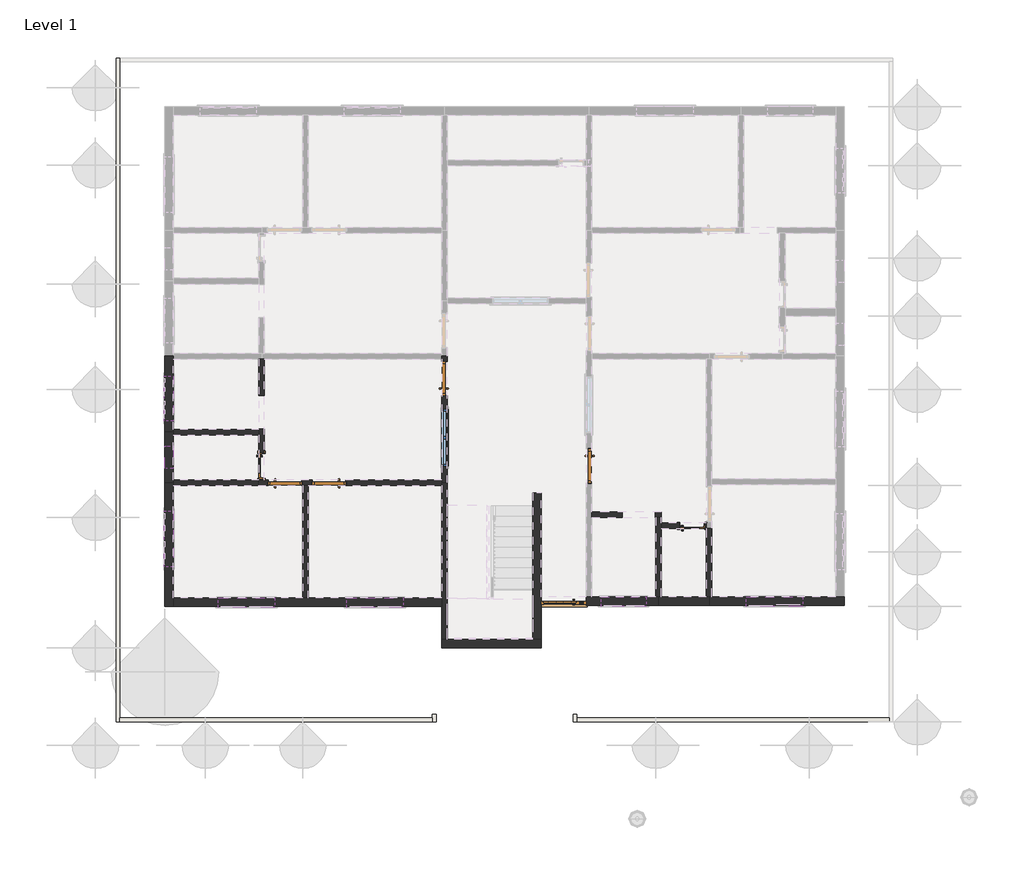
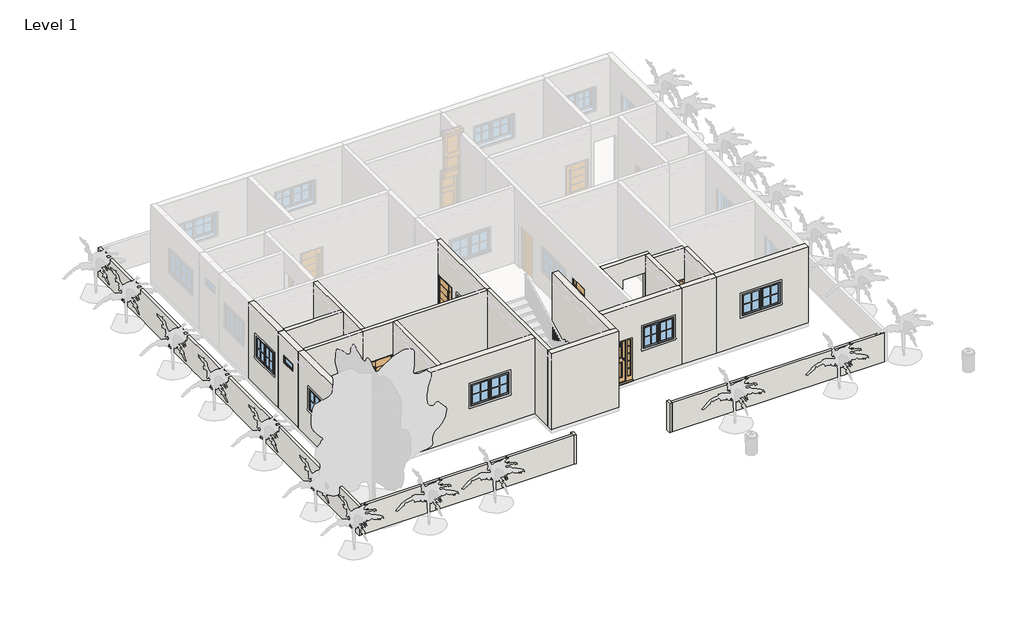
# One storey, part 1 of 5: 25 walls, 8 windows, 7 doors.
"""IFC4 building model written with IfcOpenShell, lengths in millimetres."""

from ifc_helpers import new_model, si_unit, frame, origin, origin_with_axes, place, context, project, spatial, polyline, outline, extrude, faceted_brep, transform, mapped, element, save
from components import door_3_ad1505b7, door_3_44036f4b, extsgl_w_side_panel_4_38b62cc9, door_c5a180fb, fixed_2_d9cafb20, m_window_awning_double_horizontal_4_0c6a2509, m_window_awning_double_horizontal_5_7c720334, m_window_awning_double_horizontal_5_337400f2

model = new_model("IFC4")

# Units and contexts
model_context = context("Model", 3, world=origin())
ifc_project = project(units=[si_unit("LENGTHUNIT", "METRE", prefix="MILLI")], contexts=[model_context])

# Site, building, storey
site = spatial("IfcSite", under=ifc_project)
building = spatial("IfcBuilding", under=site)
storey = spatial("IfcBuildingStorey", under=building, Name="Level 1", Elevation=0.0)

# Doors
placement = place(None, origin())
door_3_shape = door_3_ad1505b7(model_context)
element("IfcDoor", 1, ObjectType="3'", at=placement, inside=storey, context=model_context, shape_type="MappedRepresentation", body=[
    mapped(door_3_shape, transform((-17435.4847893, 15964.9922903, 0.0), x_axis=(0.0, 1.0, 0.0), y_axis=(-1.0, 0.0, 0.0), z_axis=(0.0, 0.0, 1.0))),
])
element("IfcDoor", 2, ObjectType="3'", at=placement, inside=storey, context=model_context, shape_type="MappedRepresentation", body=[
    mapped(door_3_shape, transform((-20559.6847893, 13145.5922903, 0.0), x_axis=(-1.0, 0.0, 0.0), y_axis=(0.0, -1.0, 0.0), z_axis=(0.0, 0.0, 1.0))),
])
element("IfcDoor", 3, ObjectType="3'", at=placement, inside=storey, context=model_context, shape_type="MappedRepresentation", body=[
    mapped(door_3_shape, transform((-13523.8847893, 13602.7922903, 0.0), x_axis=(0.0, -1.0, 0.0), y_axis=(1.0, 0.0, 0.0), z_axis=(0.0, 0.0, 1.0))),
])
door_3_2_shape = door_3_44036f4b(model_context)
element("IfcDoor", 4, ObjectType="3'", at=placement, inside=storey, context=model_context, shape_type="MappedRepresentation", body=[
    mapped(door_3_2_shape, transform((-21753.4847893, 13145.5922903, 0.0), x_axis=(1.0, 0.0, 0.0), y_axis=(0.0, 1.0, 0.0), z_axis=(0.0, 0.0, 1.0))),
])
extsgl_w_side_panel_4_shape = extsgl_w_side_panel_4_38b62cc9(model_context)
element("IfcDoor", 5, ObjectType="ExtSgl w Side Panel : 4'", at=placement, inside=storey, context=model_context, shape_type="MappedRepresentation", body=[
    mapped(extsgl_w_side_panel_4_shape, transform((-14429.0847893, 9932.4922903, 0.0), x_axis=(-1.0, 0.0, 0.0), y_axis=(0.0, -1.0, 0.0), z_axis=(0.0, 0.0, 1.0))),
])
door_shape = door_c5a180fb(model_context)
element("IfcDoor", 6, ObjectType="M_Door-Interior-Single-2_Panel-Wood : 2'2\"", at=placement, inside=storey, context=model_context, shape_type="MappedRepresentation", body=[
    mapped(door_shape, transform((-22391.6597893, 13602.7922903, 0.0), x_axis=(0.0, -1.0, 0.0), y_axis=(1.0, 0.0, 0.0), z_axis=(0.0, 0.0, 1.0))),
])
element("IfcDoor", 7, ObjectType="M_Door-Interior-Single-2_Panel-Wood : 2'2\"", at=placement, inside=storey, context=model_context, shape_type="MappedRepresentation", body=[
    mapped(door_shape, transform((-10729.8847893, 11974.0172903, 0.0), x_axis=(1.0, 0.0, 0.0), y_axis=(0.0, 1.0, 0.0), z_axis=(0.0, 0.0, 1.0))),
])

# Walls
element("IfcWall", 8, ObjectType="Generic - 4\"", at=placement, inside=storey, context=model_context, shape_type="Brep", body=[
    faceted_brep([(-26325.4847893, 24651.7922903, -152.4), (-26325.4847893, 6668.5922903, -152.4), (-26325.4847893, 6668.5922903, 1066.8), (-26325.4847893, 24651.7922903, 1066.8), (-26223.8847893, 24651.7922903, -152.4), (-26223.8847893, 24651.7922903, 1066.8), (-26223.8847893, 24550.1922903, 1066.8), (-26223.8847893, 6770.1922903, 1066.8), (-26223.8847893, 6668.5922903, 1066.8), (-26223.8847893, 6668.5922903, -152.4), (-26223.8847893, 6770.1922903, -152.4), (-26223.8847893, 24550.1922903, -152.4)], [[[0, 1, 2, 3]], [[4, 5, 6, 7, 8, 9, 10, 11]], [[1, 0, 4, 11, 10, 9]], [[3, 2, 8, 7, 6, 5]], [[2, 1, 9, 8]], [[0, 3, 5, 4]]]),
])
element("IfcWall", 9, ObjectType="Generic - 4\"", at=placement, inside=storey, context=model_context, shape_type="SweptSolid", body=[
    extrude(outline(polyline([(-17765.6847893, 6668.5922903), (-26223.8847893, 6668.5922903), (-26223.8847893, 6770.1922903), (-17765.6847893, 6770.1922903), (-17765.6847893, 6668.5922903)])), frame((0.0, 0.0, -152.4), z_axis=(0.0, 0.0, 1.0), x_axis=(1.0, 0.0, 0.0)), (0.0, 0.0, 1.0), 1219.2),
])
element("IfcWall", 10, ObjectType="Generic - 4\"", at=placement, inside=storey, context=model_context, shape_type="Brep", body=[
    faceted_brep([(-17664.0847893, 6668.5922903, -152.4), (-17664.0847893, 6871.7922903, -152.4), (-17664.0847893, 6871.7922903, 1066.8), (-17664.0847893, 6668.5922903, 1066.8), (-17765.6847893, 6668.5922903, -152.4), (-17765.6847893, 6668.5922903, 1066.8), (-17765.6847893, 6770.1922903, 1066.8), (-17765.6847893, 6871.7922903, 1066.8), (-17765.6847893, 6871.7922903, -152.4), (-17765.6847893, 6770.1922903, -152.4)], [[[0, 1, 2, 3]], [[4, 5, 6, 7, 8, 9]], [[1, 0, 4, 9, 8]], [[2, 1, 8, 7]], [[3, 2, 7, 6, 5]], [[0, 3, 5, 4]]]),
])
element("IfcWall", 11, ObjectType="Generic - 4\"", at=placement, inside=storey, context=model_context, shape_type="SweptSolid", body=[
    extrude(outline(polyline([(-13854.0847893, 6770.1922903), (-5395.8847893, 6770.1922903), (-5395.8847893, 6668.5922903), (-13854.0847893, 6668.5922903), (-13854.0847893, 6770.1922903)])), frame((0.0, 0.0, -152.4), z_axis=(0.0, 0.0, 1.0), x_axis=(1.0, 0.0, 0.0)), (0.0, 0.0, 1.0), 1219.2),
])
element("IfcWall", 12, ObjectType="Generic - 4\"", at=placement, inside=storey, context=model_context, shape_type="Brep", body=[
    faceted_brep([(-13955.6847893, 6871.7922903, -152.4), (-13955.6847893, 6668.5922903, -152.4), (-13955.6847893, 6668.5922903, 1066.8), (-13955.6847893, 6871.7922903, 1066.8), (-13854.0847893, 6871.7922903, -152.4), (-13854.0847893, 6871.7922903, 1066.8), (-13854.0847893, 6770.1922903, 1066.8), (-13854.0847893, 6668.5922903, 1066.8), (-13854.0847893, 6668.5922903, -152.4), (-13854.0847893, 6770.1922903, -152.4)], [[[0, 1, 2, 3]], [[4, 5, 6, 7, 8, 9]], [[1, 0, 4, 9, 8]], [[3, 2, 7, 6, 5]], [[0, 3, 5, 4]], [[2, 1, 8, 7]]]),
])
element("IfcWall", 13, ObjectType="Generic - 6\"", at=placement, inside=storey, context=model_context, shape_type="Brep", body=[
    faceted_brep([(-24776.0847893, 13069.3922903, 0.0), (-22477.3847893, 13069.3922903, 0.0), (-22477.3847893, 13069.3922903, 3200.4), (-24776.0847893, 13069.3922903, 3200.4), (-24776.0847893, 13221.7922903, 0.0), (-24776.0847893, 13221.7922903, 3200.4), (-22477.3847893, 13221.7922903, 3200.4), (-22477.3847893, 13221.7922903, 0.0), (-24776.0847893, 13145.5922903, 0.0), (-24776.0847893, 13145.5922903, 3200.4)], [[[0, 1, 2, 3]], [[4, 5, 6, 7]], [[1, 0, 8, 4, 7]], [[2, 1, 7, 6]], [[3, 2, 6, 5, 9]], [[0, 3, 9, 5, 4, 8]]]),
])
element("IfcWall", 14, ObjectType="Generic - 6\"", at=placement, inside=storey, context=model_context, shape_type="Brep", body=[
    faceted_brep([(-22464.6847893, 13221.7922903, 3200.4), (-22464.6847893, 14440.9922903, 3200.4), (-22464.6847893, 14593.3922903, 3200.4), (-22464.6847893, 16498.3922903, 3200.4), (-22464.6847893, 16498.3922903, 0.0), (-22464.6847893, 15507.100075, 0.0), (-22464.6847893, 15507.100075, 2438.4), (-22464.6847893, 14599.1617976, 2438.4), (-22464.6847893, 14599.1617976, 0.0), (-22464.6847893, 14593.3922903, 0.0), (-22464.6847893, 14440.9922903, 0.0), (-22464.6847893, 13957.9922903, 0.0), (-22464.6847893, 13957.9922903, 1853.8), (-22464.6847893, 13247.5922903, 1853.8), (-22464.6847893, 13247.5922903, 0.0), (-22464.6847893, 13221.7922903, 0.0), (-22312.2847893, 16498.3922903, 3200.4), (-22312.2847893, 13221.7922903, 3200.4), (-22312.2847893, 13221.7922903, 0.0), (-22312.2847893, 13247.5922903, 0.0), (-22312.2847893, 13247.5922903, 1853.8), (-22312.2847893, 13957.9922903, 1853.8), (-22312.2847893, 13957.9922903, 0.0), (-22312.2847893, 14599.1617976, 0.0), (-22312.2847893, 14599.1617976, 2438.4), (-22312.2847893, 15507.100075, 2438.4), (-22312.2847893, 15507.100075, 0.0), (-22312.2847893, 16498.3922903, 0.0), (-22388.4847893, 16498.3922903, 0.0), (-22388.4847893, 16498.3922903, 3200.4)], [[[0, 1, 2, 3, 4, 5, 6, 7, 8, 9, 10, 11, 12, 13, 14, 15]], [[16, 17, 18, 19, 20, 21, 22, 23, 24, 25, 26, 27]], [[18, 15, 14, 19]], [[8, 23, 22, 11, 10, 9]], [[4, 28, 27, 26, 5]], [[3, 2, 1, 0, 17, 16, 29]], [[4, 3, 29, 16, 27, 28]], [[0, 15, 18, 17]], [[13, 20, 19, 14]], [[20, 13, 12, 21]], [[21, 12, 11, 22]], [[6, 25, 24, 7]], [[25, 6, 5, 26]], [[7, 24, 23, 8]]]),
])
element("IfcWall", 15, ObjectType="Generic - 6\"", at=placement, inside=storey, context=model_context, shape_type="Brep", body=[
    faceted_brep([(-24776.0847893, 14440.9922903, 0.0), (-22464.6847893, 14440.9922903, 0.0), (-22464.6847893, 14440.9922903, 3200.4), (-24776.0847893, 14440.9922903, 3200.4), (-24776.0847893, 14593.3922903, 0.0), (-24776.0847893, 14593.3922903, 3200.4), (-22464.6847893, 14593.3922903, 3200.4), (-22464.6847893, 14593.3922903, 0.0), (-24776.0847893, 14517.1922903, 0.0), (-24776.0847893, 14517.1922903, 3200.4)], [[[0, 1, 2, 3]], [[4, 5, 6, 7]], [[1, 0, 8, 4, 7]], [[3, 2, 6, 5, 9]], [[0, 3, 9, 5, 4, 8]], [[2, 1, 7, 6]]]),
])
element("IfcWall", 16, ObjectType="Generic - 6\"", at=placement, inside=storey, context=model_context, shape_type="SweptSolid", body=[
    extrude(outline(polyline([(-21118.4847893, 13069.3922903), (-21118.4847893, 10021.3922903), (-21270.8847893, 10021.3922903), (-21270.8847893, 13069.3922903), (-21118.4847893, 13069.3922903)])), origin_with_axes(), (0.0, 0.0, 1.0), 3200.4),
])
element("IfcWall", 17, ObjectType="Generic - 6\"", at=placement, inside=storey, context=model_context, shape_type="Brep", body=[
    faceted_brep([(-11568.0847893, 12205.7922903, 0.0), (-11568.0847893, 12205.7922903, 3200.4), (-11720.4847893, 12205.7922903, 3200.4), (-13447.6847893, 12205.7922903, 3200.4), (-13447.6847893, 12205.7922903, 0.0), (-12628.6631671, 12205.7922903, 0.0), (-12628.6631671, 12205.7922903, 2438.4), (-11726.8987952, 12205.7922903, 2438.4), (-11726.8987952, 12205.7922903, 0.0), (-11720.4847893, 12205.7922903, 0.0), (-11568.0847893, 12358.1922903, 3200.4), (-11568.0847893, 12358.1922903, 0.0), (-11726.8987952, 12358.1922903, 0.0), (-11726.8987952, 12358.1922903, 2438.4), (-12628.6631671, 12358.1922903, 2438.4), (-12628.6631671, 12358.1922903, 0.0), (-13447.6847893, 12358.1922903, 0.0), (-13447.6847893, 12358.1922903, 3200.4)], [[[0, 1, 2, 3, 4, 5, 6, 7, 8, 9]], [[10, 11, 12, 13, 14, 15, 16, 17]], [[4, 16, 15, 5]], [[11, 0, 9, 8, 12]], [[3, 2, 1, 10, 17]], [[4, 3, 17, 16]], [[1, 0, 11, 10]], [[6, 14, 13, 7]], [[14, 6, 5, 15]], [[7, 13, 12, 8]]]),
])
element("IfcWall", 18, ObjectType="Generic - 6\"", at=placement, inside=storey, context=model_context, shape_type="Brep", body=[
    faceted_brep([(-11720.4847893, 12205.7922903, 0.0), (-11720.4847893, 10046.7922903, 0.0), (-11720.4847893, 10046.7922903, 3200.4), (-11720.4847893, 12205.7922903, 3200.4), (-11568.0847893, 12205.7922903, 0.0), (-11568.0847893, 12205.7922903, 3200.4), (-11568.0847893, 12053.3922903, 3200.4), (-11568.0847893, 11900.9922903, 3200.4), (-11568.0847893, 10046.7922903, 3200.4), (-11568.0847893, 10046.7922903, 0.0), (-11568.0847893, 11900.9922903, 0.0), (-11568.0847893, 12053.3922903, 0.0), (-11644.2847893, 10046.7922903, 0.0), (-11644.2847893, 10046.7922903, 3200.4)], [[[0, 1, 2, 3]], [[4, 5, 6, 7, 8, 9, 10, 11]], [[1, 0, 4, 11, 10, 9, 12]], [[3, 2, 13, 8, 7, 6, 5]], [[0, 3, 5, 4]], [[2, 1, 12, 9, 8, 13]]]),
])
element("IfcWall", 19, ObjectType="Generic - 6\"", at=placement, inside=storey, context=model_context, shape_type="Brep", body=[
    faceted_brep([(-10348.8847893, 11900.9922903, 3200.4), (-11568.0847893, 11900.9922903, 3200.4), (-11568.0847893, 11900.9922903, 0.0), (-11085.0847893, 11900.9922903, 0.0), (-11085.0847893, 11900.9922903, 1853.8), (-10374.6847893, 11900.9922903, 1853.8), (-10374.6847893, 11900.9922903, 0.0), (-10348.8847893, 11900.9922903, 0.0), (-11568.0847893, 12053.3922903, 3200.4), (-10348.8847893, 12053.3922903, 3200.4), (-10348.8847893, 12053.3922903, 0.0), (-10374.6847893, 12053.3922903, 0.0), (-10374.6847893, 12053.3922903, 1853.8), (-11085.0847893, 12053.3922903, 1853.8), (-11085.0847893, 12053.3922903, 0.0), (-11568.0847893, 12053.3922903, 0.0), (-10348.8847893, 11913.6922903, 0.0), (-10348.8847893, 11913.6922903, 3200.4)], [[[0, 1, 2, 3, 4, 5, 6, 7]], [[8, 9, 10, 11, 12, 13, 14, 15]], [[2, 15, 14, 3]], [[10, 16, 7, 6, 11]], [[1, 0, 17, 9, 8]], [[0, 7, 16, 10, 9, 17]], [[2, 1, 8, 15]], [[5, 12, 11, 6]], [[12, 5, 4, 13]], [[13, 4, 3, 14]]]),
])
element("IfcWall", 20, ObjectType="Generic - 6\"", at=placement, inside=storey, context=model_context, shape_type="Brep", body=[
    faceted_brep([(-17511.6847893, 13145.5922903, 0.0), (-17511.6847893, 13145.5922903, 3200.4), (-17511.6847893, 13221.7922903, 3200.4), (-17511.6847893, 16498.3922903, 3200.4), (-17511.6847893, 16574.5922903, 3200.4), (-17511.6847893, 16574.5922903, 0.0), (-17511.6847893, 16498.3922903, 0.0), (-17511.6847893, 16422.1922903, 0.0), (-17511.6847893, 16422.1922903, 1828.8), (-17511.6847893, 15507.7922903, 1828.8), (-17511.6847893, 15507.7922903, 0.0), (-17511.6847893, 13221.7922903, 0.0), (-17511.6847893, 13602.7922903, 1814.4), (-17511.6847893, 13602.7922903, 900.0), (-17511.6847893, 15126.7922903, 900.0), (-17511.6847893, 15126.7922903, 1814.4), (-17359.2847893, 13145.5922903, 3200.4), (-17359.2847893, 13145.5922903, 0.0), (-17359.2847893, 15507.7922903, 0.0), (-17359.2847893, 15507.7922903, 1828.8), (-17359.2847893, 16422.1922903, 1828.8), (-17359.2847893, 16422.1922903, 0.0), (-17359.2847893, 16574.5922903, 0.0), (-17359.2847893, 16574.5922903, 3200.4), (-17359.2847893, 13602.7922903, 1814.4), (-17359.2847893, 15126.7922903, 1814.4), (-17359.2847893, 15126.7922903, 900.0), (-17359.2847893, 13602.7922903, 900.0), (-17414.6847893, 16422.1922903, 0.0), (-17414.6847893, 16437.1922903, 0.0), (-17491.6847893, 16437.1922903, 0.0), (-17491.6847893, 16422.1922903, 0.0), (-17491.6847893, 15507.7922903, 0.0), (-17491.6847893, 15492.7922903, 0.0), (-17414.6847893, 15492.7922903, 0.0), (-17414.6847893, 15507.7922903, 0.0), (-17414.6847893, 15507.7922903, 1828.8), (-17414.6847893, 16422.1922903, 1828.8), (-17491.6847893, 16422.1922903, 1828.8), (-17491.6847893, 15507.7922903, 1828.8), (-17491.6847893, 15492.7922903, 1843.8), (-17491.6847893, 16437.1922903, 1843.8), (-17414.6847893, 16437.1922903, 1843.8), (-17414.6847893, 15492.7922903, 1843.8)], [[[0, 1, 2, 3, 4, 5, 6, 7, 8, 9, 10, 11], [12, 13, 14, 15]], [[16, 17, 18, 19, 20, 21, 22, 23], [24, 25, 26, 27]], [[5, 22, 21, 28, 29, 30, 31, 7, 6]], [[17, 0, 11, 10, 32, 33, 34, 35, 18]], [[1, 0, 17, 16]], [[4, 3, 2, 1, 16, 23]], [[5, 4, 23, 22]], [[19, 36, 37, 20]], [[8, 38, 39, 9]], [[20, 37, 28, 21]], [[38, 8, 7, 31]], [[36, 19, 18, 35]], [[9, 39, 32, 10]], [[40, 41, 42, 43]], [[42, 41, 30, 29]], [[37, 36, 35, 34, 43, 42, 29, 28]], [[40, 43, 34, 33]], [[39, 38, 31, 30, 41, 40, 33, 32]], [[12, 15, 25, 24]], [[15, 14, 26, 25]], [[14, 13, 27, 26]], [[13, 12, 24, 27]]]),
])
element("IfcWall", 21, ObjectType="Generic - 6\"", at=placement, inside=storey, context=model_context, shape_type="Brep", body=[
    faceted_brep([(-17511.6847893, 13145.5922903, 0.0), (-17511.6847893, 13069.3922903, 0.0), (-17511.6847893, 10021.3922903, 0.0), (-17511.6847893, 9792.7922903, 0.0), (-17511.6847893, 8903.7922903, 0.0), (-17511.6847893, 8903.7922903, 3200.4), (-17511.6847893, 9792.7922903, 3200.4), (-17511.6847893, 10021.3922903, 3200.4), (-17511.6847893, 13069.3922903, 3200.4), (-17511.6847893, 13145.5922903, 3200.4), (-17359.2847893, 13145.5922903, 0.0), (-17359.2847893, 13145.5922903, 3200.4), (-17359.2847893, 8903.7922903, 3200.4), (-17359.2847893, 8903.7922903, 0.0)], [[[0, 1, 2, 3, 4, 5, 6, 7, 8, 9]], [[10, 11, 12, 13]], [[4, 3, 2, 1, 0, 10, 13]], [[9, 8, 7, 6, 5, 12, 11]], [[0, 9, 11, 10]], [[5, 4, 13, 12]]]),
])
element("IfcWall", 22, ObjectType="Generic - 6\"", at=placement, inside=storey, context=model_context, shape_type="Brep", body=[
    faceted_brep([(-17511.6847893, 13069.3922903, 3200.4), (-21118.4847893, 13069.3922903, 3200.4), (-21270.8847893, 13069.3922903, 3200.4), (-22477.3847893, 13069.3922903, 3200.4), (-22477.3847893, 13069.3922903, 0.0), (-22210.6847893, 13069.3922903, 0.0), (-22210.6847893, 13069.3922903, 1828.8), (-21296.2847893, 13069.3922903, 1828.8), (-21296.2847893, 13069.3922903, 0.0), (-21270.8847893, 13069.3922903, 0.0), (-21118.4847893, 13069.3922903, 0.0), (-21016.8847893, 13069.3922903, 0.0), (-21016.8847893, 13069.3922903, 1828.8), (-20102.4847893, 13069.3922903, 1828.8), (-20102.4847893, 13069.3922903, 0.0), (-17511.6847893, 13069.3922903, 0.0), (-22477.3847893, 13221.7922903, 3200.4), (-22464.6847893, 13221.7922903, 3200.4), (-22312.2847893, 13221.7922903, 3200.4), (-17511.6847893, 13221.7922903, 3200.4), (-17511.6847893, 13221.7922903, 0.0), (-20102.4847893, 13221.7922903, 0.0), (-20102.4847893, 13221.7922903, 1828.8), (-21016.8847893, 13221.7922903, 1828.8), (-21016.8847893, 13221.7922903, 0.0), (-21296.2847893, 13221.7922903, 0.0), (-21296.2847893, 13221.7922903, 1828.8), (-22210.6847893, 13221.7922903, 1828.8), (-22210.6847893, 13221.7922903, 0.0), (-22312.2847893, 13221.7922903, 0.0), (-22464.6847893, 13221.7922903, 0.0), (-22477.3847893, 13221.7922903, 0.0), (-17511.6847893, 13145.5922903, 0.0), (-20102.4847893, 13089.3922903, 0.0), (-20087.4847893, 13089.3922903, 0.0), (-20087.4847893, 13166.3922903, 0.0), (-20102.4847893, 13166.3922903, 0.0), (-21296.2847893, 13089.3922903, 0.0), (-21281.2847893, 13089.3922903, 0.0), (-21281.2847893, 13166.3922903, 0.0), (-21296.2847893, 13166.3922903, 0.0), (-21016.8847893, 13166.3922903, 0.0), (-21031.8847893, 13166.3922903, 0.0), (-21031.8847893, 13089.3922903, 0.0), (-21016.8847893, 13089.3922903, 0.0), (-22210.6847893, 13166.3922903, 0.0), (-22225.6847893, 13166.3922903, 0.0), (-22225.6847893, 13089.3922903, 0.0), (-22210.6847893, 13089.3922903, 0.0), (-17511.6847893, 13145.5922903, 3200.4), (-22210.6847893, 13166.3922903, 1828.8), (-21296.2847893, 13166.3922903, 1828.8), (-22210.6847893, 13089.3922903, 1828.8), (-21296.2847893, 13089.3922903, 1828.8), (-21281.2847893, 13089.3922903, 1843.8), (-22225.6847893, 13089.3922903, 1843.8), (-22225.6847893, 13166.3922903, 1843.8), (-21281.2847893, 13166.3922903, 1843.8), (-20102.4847893, 13166.3922903, 1828.8), (-21016.8847893, 13166.3922903, 1828.8), (-21016.8847893, 13089.3922903, 1828.8), (-20102.4847893, 13089.3922903, 1828.8), (-20087.4847893, 13089.3922903, 1843.8), (-21031.8847893, 13089.3922903, 1843.8), (-21031.8847893, 13166.3922903, 1843.8), (-20087.4847893, 13166.3922903, 1843.8)], [[[0, 1, 2, 3, 4, 5, 6, 7, 8, 9, 10, 11, 12, 13, 14, 15]], [[16, 17, 18, 19, 20, 21, 22, 23, 24, 25, 26, 27, 28, 29, 30, 31]], [[20, 32, 15, 14, 33, 34, 35, 36, 21]], [[8, 37, 38, 39, 40, 25, 24, 41, 42, 43, 44, 11, 10, 9]], [[4, 31, 30, 29, 28, 45, 46, 47, 48, 5]], [[3, 2, 1, 0, 49, 19, 18, 17, 16]], [[4, 3, 16, 31]], [[0, 15, 32, 20, 19, 49]], [[50, 27, 26, 51]], [[6, 52, 53, 7]], [[51, 26, 25, 40]], [[7, 53, 37, 8]], [[27, 50, 45, 28]], [[52, 6, 5, 48]], [[54, 55, 56, 57]], [[54, 57, 39, 38]], [[57, 56, 46, 45, 50, 51, 40, 39]], [[56, 55, 47, 46]], [[55, 54, 38, 37, 53, 52, 48, 47]], [[22, 58, 59, 23]], [[12, 60, 61, 13]], [[23, 59, 41, 24]], [[60, 12, 11, 44]], [[58, 22, 21, 36]], [[13, 61, 33, 14]], [[62, 63, 64, 65]], [[64, 63, 43, 42]], [[59, 58, 36, 35, 65, 64, 42, 41]], [[62, 65, 35, 34]], [[61, 60, 44, 43, 63, 62, 34, 33]]]),
])
element("IfcWall", 23, ObjectType="Generic - 6\"", at=placement, inside=storey, context=model_context, shape_type="Brep", body=[
    faceted_brep([(-10348.8847893, 11913.6922903, 0.0), (-10348.8847893, 10046.7922903, 0.0), (-10348.8847893, 10046.7922903, 3200.4), (-10348.8847893, 11913.6922903, 3200.4), (-10196.4847893, 11913.6922903, 0.0), (-10196.4847893, 11913.6922903, 3200.4), (-10196.4847893, 10046.7922903, 3200.4), (-10196.4847893, 10046.7922903, 0.0), (-10272.6847893, 10046.7922903, 0.0), (-10272.6847893, 10046.7922903, 3200.4)], [[[0, 1, 2, 3]], [[4, 5, 6, 7]], [[1, 0, 4, 7, 8]], [[3, 2, 9, 6, 5]], [[0, 3, 5, 4]], [[2, 1, 8, 7, 6, 9]]]),
])
element("IfcWall", 24, ObjectType="Generic - 9\"", at=placement, inside=storey, context=model_context, shape_type="Brep", body=[
    faceted_brep([(-24776.0847893, 9792.7922903, 0.0), (-17511.6847893, 9792.7922903, 0.0), (-17511.6847893, 9792.7922903, 3200.4), (-24776.0847893, 9792.7922903, 3200.4), (-23556.8847893, 9792.7922903, 2133.5570313), (-22032.8847893, 9792.7922903, 2133.5570313), (-22032.8847893, 9792.7922903, 1219.1570313), (-23556.8847893, 9792.7922903, 1219.1570313), (-20077.0847893, 9792.7922903, 2133.5570313), (-18553.0847893, 9792.7922903, 2133.5570313), (-18553.0847893, 9792.7922903, 1219.1570313), (-20077.0847893, 9792.7922903, 1219.1570313), (-24776.0847893, 10021.3922903, 0.0), (-24776.0847893, 10021.3922903, 3200.4), (-21270.8847893, 10021.3922903, 3200.4), (-21118.4847893, 10021.3922903, 3200.4), (-17511.6847893, 10021.3922903, 3200.4), (-17511.6847893, 10021.3922903, 0.0), (-21118.4847893, 10021.3922903, 0.0), (-21270.8847893, 10021.3922903, 0.0), (-23556.8847893, 10021.3922903, 2133.5570313), (-23556.8847893, 10021.3922903, 1219.1570313), (-22032.8847893, 10021.3922903, 1219.1570313), (-22032.8847893, 10021.3922903, 2133.5570313), (-20077.0847893, 10021.3922903, 2133.5570313), (-20077.0847893, 10021.3922903, 1219.1570313), (-18553.0847893, 10021.3922903, 1219.1570313), (-18553.0847893, 10021.3922903, 2133.5570313)], [[[0, 1, 2, 3], [4, 5, 6, 7], [8, 9, 10, 11]], [[12, 13, 14, 15, 16, 17, 18, 19], [20, 21, 22, 23], [24, 25, 26, 27]], [[1, 0, 12, 19, 18, 17]], [[3, 2, 16, 15, 14, 13]], [[0, 3, 13, 12]], [[2, 1, 17, 16]], [[21, 20, 4, 7]], [[22, 21, 7, 6]], [[23, 22, 6, 5]], [[20, 23, 5, 4]], [[25, 24, 8, 11]], [[26, 25, 11, 10]], [[27, 26, 10, 9]], [[24, 27, 9, 8]]]),
])
element("IfcWall", 25, ObjectType="Generic - 9\"", at=placement, inside=storey, context=model_context, shape_type="Brep", body=[
    faceted_brep([(-17511.6847893, 8675.1922903, 0.0), (-14819.2847893, 8675.1922903, 0.0), (-14819.2847893, 8675.1922903, 3200.4), (-17511.6847893, 8675.1922903, 3200.4), (-17511.6847893, 8903.7922903, 0.0), (-17511.6847893, 8903.7922903, 3200.4), (-17359.2847893, 8903.7922903, 3200.4), (-15047.8847893, 8903.7922903, 3200.4), (-14819.2847893, 8903.7922903, 3200.4), (-14819.2847893, 8903.7922903, 0.0), (-15047.8847893, 8903.7922903, 0.0), (-17359.2847893, 8903.7922903, 0.0)], [[[0, 1, 2, 3]], [[4, 5, 6, 7, 8, 9, 10, 11]], [[1, 0, 4, 11, 10, 9]], [[3, 2, 8, 7, 6, 5]], [[2, 1, 9, 8]], [[0, 3, 5, 4]]]),
])
element("IfcWall", 26, ObjectType="Generic - 9\"", at=placement, inside=storey, context=model_context, shape_type="Brep", body=[
    faceted_brep([(-14819.2847893, 8903.7922903, 0.0), (-14819.2847893, 9818.1922903, 0.0), (-14819.2847893, 10046.7922903, 0.0), (-14819.2847893, 12866.1922903, 0.0), (-14819.2847893, 12866.1922903, 3200.4), (-14819.2847893, 10046.7922903, 3200.4), (-14819.2847893, 9818.1922903, 3200.4), (-14819.2847893, 8903.7922903, 3200.4), (-15047.8847893, 8903.7922903, 0.0), (-15047.8847893, 8903.7922903, 3200.4), (-15047.8847893, 12866.1922903, 3200.4), (-15047.8847893, 12866.1922903, 0.0)], [[[0, 1, 2, 3, 4, 5, 6, 7]], [[8, 9, 10, 11]], [[3, 2, 1, 0, 8, 11]], [[4, 3, 11, 10]], [[7, 6, 5, 4, 10, 9]], [[0, 7, 9, 8]]]),
])
element("IfcWall", 27, ObjectType="Generic - 9\"", at=placement, inside=storey, context=model_context, shape_type="Brep", body=[
    faceted_brep([(-6615.0847893, 10046.7922903, 0.0), (-6843.6847893, 10046.7922903, 0.0), (-10196.4847893, 10046.7922903, 0.0), (-10272.6847893, 10046.7922903, 0.0), (-10272.6847893, 10046.7922903, 3200.4), (-10196.4847893, 10046.7922903, 3200.4), (-6843.6847893, 10046.7922903, 3200.4), (-6615.0847893, 10046.7922903, 3200.4), (-9263.0347893, 10046.7922903, 2133.5570313), (-9263.0347893, 10046.7922903, 1219.1570313), (-7739.0347893, 10046.7922903, 1219.1570313), (-7739.0347893, 10046.7922903, 2133.5570313), (-6615.0847893, 9818.1922903, 0.0), (-6615.0847893, 9818.1922903, 3200.4), (-10272.6847893, 9818.1922903, 3200.4), (-10272.6847893, 9818.1922903, 0.0), (-9263.0347893, 9818.1922903, 2133.5570313), (-7739.0347893, 9818.1922903, 2133.5570313), (-7739.0347893, 9818.1922903, 1219.1570313), (-9263.0347893, 9818.1922903, 1219.1570313)], [[[0, 1, 2, 3, 4, 5, 6, 7], [8, 9, 10, 11]], [[12, 13, 14, 15], [16, 17, 18, 19]], [[3, 2, 1, 0, 12, 15]], [[4, 3, 15, 14]], [[7, 6, 5, 4, 14, 13]], [[0, 7, 13, 12]], [[9, 8, 16, 19]], [[10, 9, 19, 18]], [[11, 10, 18, 17]], [[8, 11, 17, 16]]]),
])
element("IfcWall", 28, ObjectType="Generic - 9\"", at=placement, inside=storey, context=model_context, shape_type="Brep", body=[
    faceted_brep([(-10272.6847893, 10046.7922903, 0.0), (-10348.8847893, 10046.7922903, 0.0), (-11568.0847893, 10046.7922903, 0.0), (-11644.2847893, 10046.7922903, 0.0), (-11644.2847893, 10046.7922903, 3200.4), (-11568.0847893, 10046.7922903, 3200.4), (-10348.8847893, 10046.7922903, 3200.4), (-10272.6847893, 10046.7922903, 3200.4), (-10272.6847893, 9818.1922903, 0.0), (-10272.6847893, 9818.1922903, 3200.4), (-11644.2847893, 9818.1922903, 3200.4), (-11644.2847893, 9818.1922903, 0.0)], [[[0, 1, 2, 3, 4, 5, 6, 7]], [[8, 9, 10, 11]], [[3, 2, 1, 0, 8, 11]], [[4, 3, 11, 10]], [[7, 6, 5, 4, 10, 9]], [[0, 7, 9, 8]]]),
])
element("IfcWall", 29, ObjectType="Generic - 9\"", at=placement, inside=storey, context=model_context, shape_type="Brep", body=[
    faceted_brep([(-14819.2847893, 10046.7922903, 3200.4), (-13600.0847893, 10046.7922903, 3200.4), (-13447.6847893, 10046.7922903, 3200.4), (-11720.4847893, 10046.7922903, 3200.4), (-11644.2847893, 10046.7922903, 3200.4), (-11644.2847893, 10046.7922903, 0.0), (-11720.4847893, 10046.7922903, 0.0), (-13447.6847893, 10046.7922903, 0.0), (-13600.0847893, 10046.7922903, 0.0), (-13600.0847893, 10046.7922903, 1828.8), (-14819.2847893, 10046.7922903, 1828.8), (-13193.6847893, 10046.7922903, 2133.6), (-13193.6847893, 10046.7922903, 1219.2), (-11974.4847893, 10046.7922903, 1219.2), (-11974.4847893, 10046.7922903, 2133.6), (-11644.2847893, 9818.1922903, 3200.4), (-14819.2847893, 9818.1922903, 3200.4), (-14819.2847893, 9818.1922903, 1828.8), (-13600.0847893, 9818.1922903, 1828.8), (-13600.0847893, 9818.1922903, 0.0), (-11644.2847893, 9818.1922903, 0.0), (-13193.6847893, 9818.1922903, 2133.6), (-11974.4847893, 9818.1922903, 2133.6), (-11974.4847893, 9818.1922903, 1219.2), (-13193.6847893, 9818.1922903, 1219.2)], [[[0, 1, 2, 3, 4, 5, 6, 7, 8, 9, 10], [11, 12, 13, 14]], [[15, 16, 17, 18, 19, 20], [21, 22, 23, 24]], [[5, 20, 19, 8, 7, 6]], [[4, 3, 2, 1, 0, 16, 15]], [[5, 4, 15, 20]], [[16, 0, 10, 17]], [[11, 14, 22, 21]], [[14, 13, 23, 22]], [[13, 12, 24, 23]], [[12, 11, 21, 24]], [[18, 9, 8, 19]], [[9, 18, 17, 10]]]),
])
element("IfcWall", 30, ObjectType="Generic - 9\"", at=placement, inside=storey, context=model_context, shape_type="Brep", body=[
    faceted_brep([(-25004.6847893, 16574.5922903, 0.0), (-25004.6847893, 14517.1922903, 0.0), (-25004.6847893, 14517.1922903, 3200.4), (-25004.6847893, 16574.5922903, 3200.4), (-25004.6847893, 16041.1922903, 2133.6), (-25004.6847893, 14821.9922903, 2133.6), (-25004.6847893, 14821.9922903, 1219.2), (-25004.6847893, 16041.1922903, 1219.2), (-24776.0847893, 16574.5922903, 0.0), (-24776.0847893, 16574.5922903, 3200.4), (-24776.0847893, 16498.3922903, 3200.4), (-24776.0847893, 14593.3922903, 3200.4), (-24776.0847893, 14517.1922903, 3200.4), (-24776.0847893, 14517.1922903, 0.0), (-24776.0847893, 14593.3922903, 0.0), (-24776.0847893, 16498.3922903, 0.0), (-24776.0847893, 16041.1922903, 2133.6), (-24776.0847893, 16041.1922903, 1219.2), (-24776.0847893, 14821.9922903, 1219.2), (-24776.0847893, 14821.9922903, 2133.6)], [[[0, 1, 2, 3], [4, 5, 6, 7]], [[8, 9, 10, 11, 12, 13, 14, 15], [16, 17, 18, 19]], [[1, 0, 8, 15, 14, 13]], [[2, 1, 13, 12]], [[3, 2, 12, 11, 10, 9]], [[0, 3, 9, 8]], [[16, 19, 5, 4]], [[19, 18, 6, 5]], [[18, 17, 7, 6]], [[17, 16, 4, 7]]]),
])
element("IfcWall", 31, ObjectType="Generic - 9\"", at=placement, inside=storey, context=model_context, shape_type="Brep", body=[
    faceted_brep([(-25004.6847893, 14517.1922903, 0.0), (-25004.6847893, 13145.5922903, 0.0), (-25004.6847893, 13145.5922903, 3200.4), (-25004.6847893, 14517.1922903, 3200.4), (-25004.6847893, 14136.1922903, 2438.4), (-25004.6847893, 13526.5922903, 2438.4), (-25004.6847893, 13526.5922903, 2133.6), (-25004.6847893, 14136.1922903, 2133.6), (-24776.0847893, 14517.1922903, 0.0), (-24776.0847893, 14517.1922903, 3200.4), (-24776.0847893, 14440.9922903, 3200.4), (-24776.0847893, 13221.7922903, 3200.4), (-24776.0847893, 13145.5922903, 3200.4), (-24776.0847893, 13145.5922903, 0.0), (-24776.0847893, 13221.7922903, 0.0), (-24776.0847893, 14440.9922903, 0.0), (-24776.0847893, 14136.1922903, 2438.4), (-24776.0847893, 14136.1922903, 2133.6), (-24776.0847893, 13526.5922903, 2133.6), (-24776.0847893, 13526.5922903, 2438.4)], [[[0, 1, 2, 3], [4, 5, 6, 7]], [[8, 9, 10, 11, 12, 13, 14, 15], [16, 17, 18, 19]], [[1, 0, 8, 15, 14, 13]], [[2, 1, 13, 12]], [[3, 2, 12, 11, 10, 9]], [[0, 3, 9, 8]], [[16, 19, 5, 4]], [[19, 18, 6, 5]], [[18, 17, 7, 6]], [[17, 16, 4, 7]]]),
])
element("IfcWall", 32, ObjectType="Generic - 9\"", at=placement, inside=storey, context=model_context, shape_type="Brep", body=[
    faceted_brep([(-25004.6847893, 13145.5922903, 0.0), (-25004.6847893, 9792.7922903, 0.0), (-25004.6847893, 9792.7922903, 3200.4), (-25004.6847893, 13145.5922903, 3200.4), (-25004.6847893, 12383.5922903, 2133.5570313), (-25004.6847893, 10859.5922903, 2133.5570313), (-25004.6847893, 10859.5922903, 1219.1570313), (-25004.6847893, 12383.5922903, 1219.1570313), (-24776.0847893, 13145.5922903, 0.0), (-24776.0847893, 13145.5922903, 3200.4), (-24776.0847893, 13069.3922903, 3200.4), (-24776.0847893, 10021.3922903, 3200.4), (-24776.0847893, 9792.7922903, 3200.4), (-24776.0847893, 9792.7922903, 0.0), (-24776.0847893, 10021.3922903, 0.0), (-24776.0847893, 13069.3922903, 0.0), (-24776.0847893, 12383.5922903, 2133.5570313), (-24776.0847893, 12383.5922903, 1219.1570313), (-24776.0847893, 10859.5922903, 1219.1570313), (-24776.0847893, 10859.5922903, 2133.5570313)], [[[0, 1, 2, 3], [4, 5, 6, 7]], [[8, 9, 10, 11, 12, 13, 14, 15], [16, 17, 18, 19]], [[1, 0, 8, 15, 14, 13]], [[3, 2, 12, 11, 10, 9]], [[0, 3, 9, 8]], [[2, 1, 13, 12]], [[16, 19, 5, 4]], [[19, 18, 6, 5]], [[18, 17, 7, 6]], [[17, 16, 4, 7]]]),
])

# Windows
fixed_2_shape = fixed_2_d9cafb20(model_context)
element("IfcWindow", 33, ObjectType="Fixed : 2'", at=placement, inside=storey, context=model_context, shape_type="MappedRepresentation", body=[
    mapped(fixed_2_shape, transform((-24890.3847893, 13869.4922903, 0.0), x_axis=(0.0, 1.0, 0.0), y_axis=(-1.0, 0.0, 0.0), z_axis=(0.0, 0.0, 1.0))),
])
m_window_awning_double_horizontal_4_shape = m_window_awning_double_horizontal_4_0c6a2509(model_context)
element("IfcWindow", 34, ObjectType="M_Window-Awning-Double-Horizontal : 4'", at=placement, inside=storey, context=model_context, shape_type="MappedRepresentation", body=[
    mapped(m_window_awning_double_horizontal_4_shape, transform((-24890.3847893, 15431.5922903, 319.2), x_axis=(0.0, 1.0, 0.0), y_axis=(-1.0, 0.0, 0.0), z_axis=(0.0, 0.0, 1.0))),
])
element("IfcWindow", 35, ObjectType="M_Window-Awning-Double-Horizontal : 4'", at=placement, inside=storey, context=model_context, shape_type="MappedRepresentation", body=[
    mapped(m_window_awning_double_horizontal_4_shape, transform((-12584.0847893, 9932.4922903, 319.2), x_axis=(-1.0, 0.0, 0.0), y_axis=(0.0, -1.0, 0.0), z_axis=(0.0, 0.0, 1.0))),
])
m_window_awning_double_horizontal_5_shape = m_window_awning_double_horizontal_5_7c720334(model_context)
element("IfcWindow", 36, ObjectType="M_Window-Awning-Double-Horizontal : 5'", at=placement, inside=storey, context=model_context, shape_type="MappedRepresentation", body=[
    mapped(m_window_awning_double_horizontal_5_shape, transform((-24890.3847893, 11621.5922903, 319.1570312), x_axis=(0.0, 1.0, 0.0), y_axis=(-1.0, 0.0, 0.0), z_axis=(0.0, 0.0, 1.0))),
])
element("IfcWindow", 37, ObjectType="M_Window-Awning-Double-Horizontal : 5'", at=placement, inside=storey, context=model_context, shape_type="MappedRepresentation", body=[
    mapped(m_window_awning_double_horizontal_5_shape, transform((-22794.8847893, 9907.0922903, 319.1570312), x_axis=(-1.0, 0.0, 0.0), y_axis=(0.0, -1.0, 0.0), z_axis=(0.0, 0.0, 1.0))),
])
element("IfcWindow", 38, ObjectType="M_Window-Awning-Double-Horizontal : 5'", at=placement, inside=storey, context=model_context, shape_type="MappedRepresentation", body=[
    mapped(m_window_awning_double_horizontal_5_shape, transform((-19315.0847893, 9907.0922903, 319.1570312), x_axis=(-1.0, 0.0, 0.0), y_axis=(0.0, -1.0, 0.0), z_axis=(0.0, 0.0, 1.0))),
])
element("IfcWindow", 39, ObjectType="M_Window-Awning-Double-Horizontal : 5'", at=placement, inside=storey, context=model_context, shape_type="MappedRepresentation", body=[
    mapped(m_window_awning_double_horizontal_5_shape, transform((-8501.0347893, 9932.4922903, 319.1570312), x_axis=(-1.0, 0.0, 0.0), y_axis=(0.0, -1.0, 0.0), z_axis=(0.0, 0.0, 1.0))),
])
m_window_awning_double_horizontal_5_2_shape = m_window_awning_double_horizontal_5_337400f2(model_context)
element("IfcWindow", 40, ObjectType="M_Window-Awning-Double-Horizontal : 5'", at=placement, inside=storey, context=model_context, shape_type="MappedRepresentation", body=[
    mapped(m_window_awning_double_horizontal_5_2_shape, transform((-17435.4847893, 14364.7922903, 0.0), x_axis=(0.0, -1.0, 0.0), y_axis=(1.0, 0.0, 0.0), z_axis=(0.0, 0.0, 1.0))),
])

save(model, "model.ifc")

# Revit data of these elements
# Type "3'"
#   Type Mark = "9"
#   Water resistance = "up to Class E900, EN 12208:2001"
#   Uniclass2015Version = "v1.21"
#   Uniclass2015Reference = "Ss_25_30_20_30"
#   Uniclass2015Description = "Frame and door leaf system"
#   URL = "www.aluprof.com"
#   Type IFC Predefined Type = "USERDEFINED"
#   Right-hand / Left-hand door [instance default] = ""
#   Resistance to wind load = "up to Class C5/B5, EN 12210:2001"
#   Insert type = "ST"
#   Hardware [instance default] = ""
#   Product page = "https://aluprof.com/en/architects/offer/window-and-door-systems/panel-doors#visualisation"
#   Operation = "SinglePanelOutwardOpening"
#   Opening type = "Outward"
#   NBSReference = "25-50-20/125"
#   NBSDescription = "Frame and door leaf system"
#   Important = "The actual acceptable construction dimensions are dependent on the selection of profiles and hardware, glazing type, construction weight and the construction’s operating conditions. These should be determined by a suitably qualified person, and using ALUPROF’s calculation software"
#   IfcExportType = "USERDEFINED"
#   IfcExportAs = "IfcDoorType"
#   Handle type [instance default] = ""
#   Manufacturer = "ALUPROF SA"
#   Export Type to IFC As = "IfcDoorType"
#   Door sill type [instance default] = ""
#   Description = "External single-leaf panel door outward opening"
#   Model = "MB-86 ST Panel Door AD07"
#   Content of the recyclate in the material = "69.2%"
#   COBie.Type.WarrantyDurationParts = ""
#   COBie.Type.Name = ""
#   COBie.Type.Manufacturer = "ALUPROF SA"
#   COBie.Space.Name = ""
#   COBie.Floor.Name = ""
#   COBie.Facility.Name = ""
#   COBie.CreatedOn = ""
#   COBie.Component.WarrantyStartDate = ""
#   COBie.Component.Name = "MB-86 ST Panel Door AD07"
#   Burglar resistance = "RC2"
#   Air permeability = "up to Class 4, EN 12207:2001"
#   Width of the active leaf = 2' - 8.17717"
#   Placement in wall = 0' - 0.7874"
#   Thickness = 0' - 3.0315"
#   Height of the opening sash = 5' - 9.44094"
#   Handle Offset = 3' - 5.33858"
#   Rough Height = 6' - 2.40945"
#   Rough Width = 3' - 1.1811"
#   Height = 6' - 0"
#   Width = 3' - 0"
#   Construction depth = 0' - 3.0315"
#   Clear opening width = 2' - 3.94882"
#   Clear opening height = 5' - 8.47638"
#   Height of the array = 0' - 11.08136"
#   Schedule No. [instance default] = 1
#   Handrail [instance default] = yes
#   IsExternal = yes
#   Handle [instance default] = no
#   Door closer [instance default] = no
#   Function = 1
#   COBie.Type = yes
#   COBie = yes
#   Access control [instance default] = no
#   Panel = element 380783
#   Wall Closure = (empty or 0)
# Type "ExtSgl w Side Panel : 4'"
#   Type Mark = "14"
#   Operation = "SingleSwingRight"
#   Keynote = "L20"
#   Wrap Layers (Int) from Ext = 0' - 6.98819"
#   Wrap Layers (Ext) from Ext = 0' - 4.03543"
#   Thickness = 0' - 1.73228"
#   Stile Top of Lock rail = 3' - 3.37008"
#   Stile Top of Frieze Rail = 5' - 3.97638"
#   Stile Top Rail = 0' - 5.90551"
#   Stile Shutting = 0' - 4.92126"
#   Panelling Widths = 0' - 9.84252"
#   Stile Lock Rail = 0' - 6.88976"
#   Stile Intermediate/Frieze = 0' - 4.92126"
#   Stile Hanging = 0' - 4.92126"
#   Stile Bottom Rail = 0' - 6.88976"
#   Rough Width = 4' - 0"
#   Rough Height = 6' - 0"
#   O/A Frame Width = 0' - 2.51969"
#   Handle Z Distance = 3' - 3.37008"
#   Glazing Thickness = 0' - 0.94488"
#   Glazing Bar Thickness = 0' - 0.98425"
#   FrameWidth = 0' - 1.65354"
#   FrameOffset - External = 0' - 0.98425"
#   FrameDepth = 0' - 3.50394"
#   Door Panel Width = 2' - 11.70866"
#   Door Panel Thickness = 0' - 1.73228"
#   Door Panel Height = 5' - 7.66929"
#   Cill Thickness = 0' - 2.14567"
#   Cill Projection = 0' - 1.1811"
#   Handle X Distance = 0' - 2.95276"
#   Height = 6' - 0"
#   Structural Tolerance = 0' - 0.25591"
#   Tolerance = 0' - 0.11811"
#   Undercut = 0' - 0.15748"
#   Width = 4' - 0"
#   Cill Extension = 0' - 0.98425"
#   Cavity Closer Width = 0' - 1.9685"
#   Cavity Closer Offset from Ext = 0' - 4.03543"
#   Cavity Closer Depth = 0' - 3.34646"
#   Vis - SideLight Glazing Bars = yes
#   Vis - Ironmongery = yes
#   Vis - Cavity Closers = yes
#   Function = 1
#   Material Glass = Door - Glazing
#   Handle Style = element 387737
#   Material Door = Door - Panel
#   Material Ironmongery = Door - Handle
#   Wall Closure = (empty or 0)
# Type "M_Door-Interior-Single-2_Panel-Wood : 2'2\""
#   Type Mark = "11"
#   Assembly Code = "C1020300"
#   Analytic Construction = "Wooden"
#   Top Rail = 0' - 4.72441"
#   Thickness = 0' - 1.37795"
#   Thermal Resistance (R) = 2.5876 (h·ft²·°F)/BTU
#   Swing Angle [instance default] = 90.00°
#   Stiles = 0' - 4.72441"
#   Rough Width = 2' - 3.9685"
#   Rough Height = 6' - 0.98425"
#   Lock Rail = 0' - 7.87402"
#   Height = 6' - 0"
#   Width = 2' - 2"
#   Heat Transfer Coefficient (U) = 0.3865 BTU/(h·ft²·°F)
#   Bottom Rail = 0' - 9.05512"
#   Trim Material = Cherry
#   Panel Material = Cherry
#   Frame Material = Cherry
#   Door Handle Material = Aluminum
#   Visual Light Transmittance = 0
#   Solar Heat Gain Coefficient = 0
#   Wall Closure = (empty or 0)
#   Function = (empty or 0)
# Type "Generic - 4\""
#   Assembly Code = "B2010"
#   Layers, outside or top first: 0' - 4" no material (function 1)
# Type "Generic - 6\""
#   Assembly Code = "B2010"
#   Layers, outside or top first: 0' - 6" no material (function 1)
# Type "Generic - 9\""
#   Assembly Code = "B2010"
#   Layers, outside or top first: 0' - 9" no material (function 1)
# Type "Fixed : 2'"
#   Type Mark = "22"
#   Construction Type Id = "GSP4R"
#   Assembly Code = "B2020100"
#   Analytic Construction = "1/8 in Pilkington single glazing"
#   Visual Light Transmittance = 0.9
#   Solar Heat Gain Coefficient = 0.78
#   Heat Transfer Coefficient (U) = 0.6496 BTU/(h·ft²·°F)
#   Height = 1' - 0"
#   Default Sill Height = 7' - 0"
#   Width = 2' - 0"
#   Window Inset = 0' - 0 3/4"
#   Define Thermal Properties by = 1
#   Glass Pane Material = Glass
#   Sash Material = Sash
#   Wall Closure = (empty or 0)
# Type "M_Window-Awning-Double-Horizontal : 4'"
#   Type Mark = "21"
#   Fire Rating = "0.5h"
#   Assembly Code = "B2020100"
#   Analytic Construction = "Double glazing - domestic"
#   Window Inset [instance default] = 0' - 0"
#   Wall Thickness [instance default] = 0' - 5.90551"
#   Interior Wall Closure [instance default] = 0' - 2.15551"
#   Half Width = 2' - 0"
#   Visual Light Transmittance = 0.81
#   Thermal Resistance (R) = 1.8146 (h·ft²·°F)/BTU
#   Solar Heat Gain Coefficient = 0.76
#   Rough Width = 4' - 0.59055"
#   Rough Height = 3' - 0.59055"
#   Height = 3' - 0"
#   Heat Transfer Coefficient (U) = 0.5511 BTU/(h·ft²·°F)
#   Frame Extension [instance default] = 0' - 0 1/4"
#   Exterior Wall Closure [instance default] = 0' - 1 1/4"
#   Extension Jamb [instance default] = 0' - 2.15551"
#   Default Sill Height = 2' - 11.43307"
#   Width = 4' - 0"
#   Muntin Visibility = yes
#   Interior Trim Visibility [instance default] = yes
#   Exterior Trim Visibility [instance default] = yes
#   Extension Jamb Visibility [instance default] = yes
#   Interior Trim Material = Wood - Stained
#   Muntin Pattern = M_Muntin Pattern_2x2 : M_Muntin Pattern_2x2
#   Interior Trim = M_Trim-Window-Interior-Flat : Picture Frame
#   Interior Frame Material = Wood - Stained
#   Glass Panel Material = Glass
#   Exterior Trim Material = Clad - White
#   Exterior Trim = M_Trim-Window-Exterior-Flat : with Sill
#   Exterior Frame Material = Clad - White
#   Wall Closure = (empty or 0)
# Type "M_Window-Awning-Double-Horizontal : 5'"
#   Type Mark = "19"
#   Fire Rating = "0.5h"
#   Assembly Code = "B2020100"
#   Analytic Construction = "Double glazing - domestic"
#   Window Inset [instance default] = 0' - 0"
#   Wall Thickness [instance default] = 0' - 5.90551"
#   Interior Wall Closure [instance default] = 0' - 2.15551"
#   Half Width = 2' - 6"
#   Visual Light Transmittance = 0.81
#   Thermal Resistance (R) = 1.8146 (h·ft²·°F)/BTU
#   Solar Heat Gain Coefficient = 0.76
#   Rough Width = 5' - 0.59055"
#   Rough Height = 3' - 0.59055"
#   Height = 3' - 0"
#   Heat Transfer Coefficient (U) = 0.5511 BTU/(h·ft²·°F)
#   Frame Extension [instance default] = 0' - 0 1/4"
#   Exterior Wall Closure [instance default] = 0' - 1 1/4"
#   Extension Jamb [instance default] = 0' - 2.15551"
#   Default Sill Height = 2' - 11.43307"
#   Width = 5' - 0"
#   Muntin Visibility = yes
#   Interior Trim Visibility [instance default] = yes
#   Exterior Trim Visibility [instance default] = yes
#   Extension Jamb Visibility [instance default] = yes
#   Interior Trim Material = Wood - Stained
#   Muntin Pattern = M_Muntin Pattern_2x2 : M_Muntin Pattern_2x2
#   Interior Trim = M_Trim-Window-Interior-Flat : Picture Frame
#   Interior Frame Material = Wood - Stained
#   Glass Panel Material = Glass
#   Exterior Trim Material = Clad - White
#   Exterior Trim = M_Trim-Window-Exterior-Flat : with Sill
#   Exterior Frame Material = Clad - White
#   Wall Closure = (empty or 0)
# Elements 1, 2, 3, 4 (IfcDoor, "3'")
#   Right-hand / Left-hand door = ""
#   Hardware = ""
#   Handle type = ""
#   Door sill type = ""
#   Schedule No. = 1
#   Handrail = yes
#   Handle = no
#   Door closer = no
#   Access control = no
#   Phase Created = New Construction
# Element 5 (IfcDoor, "ExtSgl w Side Panel : 4'")
#   Phase Created = New Construction
#   Materials on its faces: "Door - Panel", "Door - Handle", "Door - Glazing"
# Elements 6, 7 (IfcDoor, "M_Door-Interior-Single-2_Panel-Wood : 2'2\"")
#   Swing Angle = 90.00°
#   Phase Created = New Construction
#   Materials on its faces: "Cherry", "Aluminum"
# Elements 8, 9, 10, 11, 12 (IfcWall, "Generic - 4\"")
#   built-in parameter 1001111 = -0' - 6"
#   Top Offset = 0' - 0"
#   Base Offset = -0' - 6"
#   Unconnected Height = 4' - 0"
#   wall height = 4' - 0"
#   Phase Created = New Construction
#   Base Constraint = Level 1
#   Materials on its faces: "Default Wall"
# Element 13 (IfcWall, "Generic - 6\"")
#   Top Offset = 0' - 0"
#   Base Offset = 0' - 0"
#   Unconnected Height = 10' - 6"
#   wall height = 10' - 6"
#   Phase Created = New Construction
#   Base Constraint = Level 1
#   Materials on its faces: "Default Wall", "BRW3"
# Element 14 (IfcWall, "Generic - 6\"")
#   Top Offset = 0' - 0"
#   Base Offset = 0' - 0"
#   Unconnected Height = 10' - 6"
#   wall height = 10' - 6"
#   Phase Created = New Construction
#   Base Constraint = Level 1
#   Materials on its faces: "Default Wall", "KW1"
# Element 15 (IfcWall, "Generic - 6\"")
#   Top Offset = 0' - 0"
#   Base Offset = 0' - 0"
#   Unconnected Height = 10' - 6"
#   wall height = 10' - 6"
#   Phase Created = New Construction
#   Base Constraint = Level 1
#   Materials on its faces: "Default Wall", "BW1", "KW1"
# Element 16 (IfcWall, "Generic - 6\"")
#   Top Offset = 0' - 0"
#   Base Offset = 0' - 0"
#   Unconnected Height = 10' - 6"
#   wall height = 10' - 6"
#   Phase Created = New Construction
#   Base Constraint = Level 1
#   Materials on its faces: "Default Wall", "BRW3", "BRW4"
# Elements 17, 19 (IfcWall, "Generic - 6\"")
#   Top Offset = 0' - 0"
#   Base Offset = 0' - 0"
#   Unconnected Height = 10' - 6"
#   wall height = 10' - 6"
#   Phase Created = New Construction
#   Base Constraint = Level 1
#   Materials on its faces: "Default Wall", "LVW2"
# Element 18 (IfcWall, "Generic - 6\"")
#   Top Offset = 0' - 0"
#   Base Offset = 0' - 0"
#   Unconnected Height = 10' - 6"
#   wall height = 10' - 6"
#   Phase Created = New Construction
#   Base Constraint = Level 1
#   Materials on its faces: "Default Wall", "KW2"
# Element 20 (IfcWall, "Generic - 6\"")
#   Top Offset = 0' - 0"
#   Base Offset = 0' - 0"
#   Unconnected Height = 10' - 6"
#   wall height = 10' - 6"
#   Phase Created = New Construction
#   Base Constraint = Level 1
#   Materials on its faces: "Default Wall", "LVW1", "LVW2"
# Element 21 (IfcWall, "Generic - 6\"")
#   Top Offset = 0' - 0"
#   Base Offset = 0' - 0"
#   Unconnected Height = 10' - 6"
#   wall height = 10' - 6"
#   Phase Created = New Construction
#   Base Constraint = Level 1
#   Materials on its faces: "Default Wall", "OW1", "LVW2"
# Element 22 (IfcWall, "Generic - 6\"")
#   Top Offset = 0' - 0"
#   Base Offset = 0' - 0"
#   Unconnected Height = 10' - 6"
#   wall height = 10' - 6"
#   Phase Created = New Construction
#   Base Constraint = Level 1
#   Materials on its faces: "Default Wall", "BRW3", "LVW1"
# Element 23 (IfcWall, "Generic - 6\"")
#   Top Offset = 0' - 0"
#   Base Offset = 0' - 0"
#   Unconnected Height = 10' - 6"
#   wall height = 10' - 6"
#   Phase Created = New Construction
#   Base Constraint = Level 1
#   Materials on its faces: "Default Wall", "BW1", "BRW4"
# Elements 24, 27 (IfcWall, "Generic - 9\"")
#   Top Offset = 0' - 0"
#   Base Offset = 0' - 0"
#   Unconnected Height = 10' - 6"
#   wall height = 10' - 6"
#   Phase Created = New Construction
#   Base Constraint = Level 1
#   Materials on its faces: "Default Wall", "OW1", "BRW4"
# Element 25 (IfcWall, "Generic - 9\"")
#   Top Offset = 0' - 0"
#   Base Offset = 0' - 0"
#   Unconnected Height = 10' - 6"
#   wall height = 10' - 6"
#   Phase Created = New Construction
#   Base Constraint = Level 1
#   Materials on its faces: "OW1", "Default Wall", "LVW2"
# Element 26 (IfcWall, "Generic - 9\"")
#   Top Offset = 0' - 0"
#   Base Offset = 0' - 0"
#   Unconnected Height = 10' - 6"
#   wall height = 10' - 6"
#   Phase Created = New Construction
#   Base Constraint = Level 1
#   Materials on its faces: "Default Wall", "OW1"
# Element 28 (IfcWall, "Generic - 9\"")
#   Top Offset = 0' - 0"
#   Base Offset = 0' - 0"
#   Unconnected Height = 10' - 6"
#   wall height = 10' - 6"
#   Phase Created = New Construction
#   Base Constraint = Level 1
#   Materials on its faces: "Default Wall", "BW1", "OW1"
# Element 29 (IfcWall, "Generic - 9\"")
#   Top Offset = 0' - 0"
#   Base Offset = 0' - 0"
#   Unconnected Height = 10' - 6"
#   wall height = 10' - 6"
#   Phase Created = New Construction
#   Base Constraint = Level 1
#   Materials on its faces: "Default Wall", "LVW2", "OW1"
# Element 30 (IfcWall, "Generic - 9\"")
#   Top Offset = 0' - 0"
#   Base Offset = 0' - 0"
#   Unconnected Height = 10' - 6"
#   wall height = 10' - 6"
#   Phase Created = New Construction
#   Base Constraint = Level 1
#   Materials on its faces: "Default Wall", "OW1", "KW2"
# Element 31 (IfcWall, "Generic - 9\"")
#   Top Offset = 0' - 0"
#   Base Offset = 0' - 0"
#   Unconnected Height = 10' - 6"
#   wall height = 10' - 6"
#   Phase Created = New Construction
#   Base Constraint = Level 1
#   Materials on its faces: "Default Wall", "OW1", "BW1"
# Element 32 (IfcWall, "Generic - 9\"")
#   Top Offset = 0' - 0"
#   Base Offset = 0' - 0"
#   Unconnected Height = 10' - 6"
#   wall height = 10' - 6"
#   Phase Created = New Construction
#   Base Constraint = Level 1
#   Materials on its faces: "Default Wall", "OW1", "BRW3"
# Element 33 (IfcWindow, "Fixed : 2'")
#   Mark = "20"
#   Phase Created = New Construction
#   Materials on its faces: "Sash", "Glass"
# Element 34 (IfcWindow, "M_Window-Awning-Double-Horizontal : 4'")
#   Mark = "12"
#   Window Inset = 0' - 0"
#   Interior Wall Closure = 0' - 2.15551"
#   Frame Extension = 0' - 0 1/4"
#   Exterior Wall Closure = 0' - 1 1/4"
#   Interior Trim Visibility = yes
#   Exterior Trim Visibility = yes
#   Phase Created = New Construction
#   Materials on its faces: "Wood - Stained", "Glass", "Clad - White"
# Element 35 (IfcWindow, "M_Window-Awning-Double-Horizontal : 4'")
#   Mark = "13"
#   Window Inset = 0' - 0"
#   Interior Wall Closure = 0' - 2.15551"
#   Frame Extension = 0' - 0 1/4"
#   Exterior Wall Closure = 0' - 1 1/4"
#   Interior Trim Visibility = yes
#   Exterior Trim Visibility = yes
#   Phase Created = New Construction
#   Materials on its faces: "Wood - Stained", "Glass", "Clad - White"
# Element 36 (IfcWindow, "M_Window-Awning-Double-Horizontal : 5'")
#   Mark = "3"
#   Window Inset = 0' - 0"
#   Interior Wall Closure = 0' - 2 5/32"
#   Frame Extension = 0' - 0 1/4"
#   Exterior Wall Closure = 0' - 1 1/4"
#   Interior Trim Visibility = yes
#   Exterior Trim Visibility = yes
#   Phase Created = New Construction
#   Materials on its faces: "Wood - Stained", "Glass", "Clad - White"
# Element 37 (IfcWindow, "M_Window-Awning-Double-Horizontal : 5'")
#   Mark = "4"
#   Window Inset = 0' - 0"
#   Interior Wall Closure = 0' - 2 5/32"
#   Frame Extension = 0' - 0 1/4"
#   Exterior Wall Closure = 0' - 1 1/4"
#   Interior Trim Visibility = yes
#   Exterior Trim Visibility = yes
#   Phase Created = New Construction
#   Materials on its faces: "Wood - Stained", "Glass", "Clad - White"
# Element 38 (IfcWindow, "M_Window-Awning-Double-Horizontal : 5'")
#   Mark = "5"
#   Window Inset = 0' - 0"
#   Interior Wall Closure = 0' - 2 5/32"
#   Frame Extension = 0' - 0 1/4"
#   Exterior Wall Closure = 0' - 1 1/4"
#   Interior Trim Visibility = yes
#   Exterior Trim Visibility = yes
#   Phase Created = New Construction
#   Materials on its faces: "Wood - Stained", "Glass", "Clad - White"
# Element 39 (IfcWindow, "M_Window-Awning-Double-Horizontal : 5'")
#   Mark = "6"
#   Window Inset = 0' - 0"
#   Interior Wall Closure = 0' - 2 5/32"
#   Frame Extension = 0' - 0 1/4"
#   Exterior Wall Closure = 0' - 1 1/4"
#   Interior Trim Visibility = yes
#   Exterior Trim Visibility = yes
#   Phase Created = New Construction
#   Materials on its faces: "Wood - Stained", "Glass", "Clad - White"
# Element 40 (IfcWindow, "M_Window-Awning-Double-Horizontal : 5'")
#   Mark = "17"
#   Window Inset = 0' - 0"
#   Interior Wall Closure = 0' - 2.15551"
#   Frame Extension = 0' - 0 1/4"
#   Exterior Wall Closure = 0' - 1 1/4"
#   Interior Trim Visibility = yes
#   Exterior Trim Visibility = yes
#   Phase Created = New Construction
#   Materials on its faces: "Wood - Stained", "Glass", "Clad - White"
# Materials
#   "Door - Glazing": colour RGB 0 0 255, transparency 0.75
#   "Door - Panel": class "Wood", colour RGB 210 159 95, transparency 0, Cost = 0
#   "Door - Handle": colour RGB 246 240 166, transparency 0
#   "Cherry": class "Wood", colour RGB 226 177 128, transparency 0, Description = "Prunus Serotina", Cost = 0
#   "Aluminum": class "Metal", colour RGB 247 247 247, transparency 0, Description = "Aluminum 6061", Cost = 0
#   "Glass": class "Glass", colour RGB 0 128 192, transparency 0.75, Description = "Soda Lime Glass", Cost = 0
#   "Sash": class "Wood", colour RGB 224 178 126, transparency 0, Cost = 0
#   "Wood - Stained": class "Wood", colour RGB 224 178 126, transparency 0, Cost = 0
#   "Clad - White": class "Wood", colour RGB 242 242 238, transparency 0, Cost = 0
#   "Default Wall": colour RGB 128 128 128, transparency 0, Cost = 0
#   "BRW3": class "Generic", colour RGB 120 120 120, transparency 0, Cost = 0
#   "KW1": class "Generic", colour RGB 120 120 120, transparency 0, Cost = 0
#   "BW1": class "Generic", colour RGB 120 120 120, transparency 0, Cost = 0
#   "BRW4": class "Generic", colour RGB 120 120 120, transparency 0, Cost = 0
#   "LVW2": class "Generic", colour RGB 120 120 120, transparency 0, Cost = 0
#   "KW2": class "Generic", colour RGB 120 120 120, transparency 0, Cost = 0
#   "LVW1": class "Generic", colour RGB 120 120 120, transparency 0, Cost = 0
#   "OW1": class "Generic", colour RGB 120 120 120, transparency 0, Cost = 0
